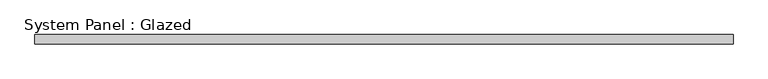
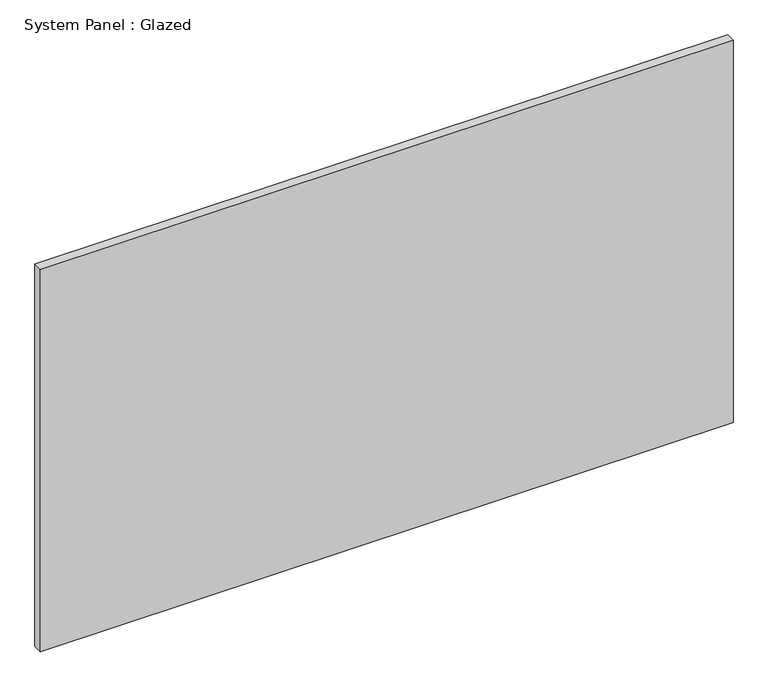
"""IFC4 building model written with IfcOpenShell, lengths in millimetres: plate geometry, System Panel : Glazed."""

from ifc_helpers import new_model, si_unit, origin, origin_with_axes, place, context, project, spatial, polyline, outline, extrude, source, transform, mapped, element, save


def system_panel_glazed_aa91312f(model_context):
    return source(origin(), model_context, "Body", "SweptSolid", [
        extrude(outline(polyline([(913.7999998, 24.5), (-913.7999998, 24.5), (-913.7999998, 49.5), (913.7999998, 49.5), (913.7999998, 24.5)])), origin_with_axes(), (0.0, 0.0, 1.0), 1066.8),
    ])


if __name__ == "__main__":
    model = new_model("IFC4")
    model_context = context("Model", 3, world=origin())
    ifc_project = project(units=[si_unit("LENGTHUNIT", "METRE", prefix="MILLI")], contexts=[model_context])
    site = spatial("IfcSite", under=ifc_project)
    building = spatial("IfcBuilding", under=site)
    placement = place(None, origin())
    system_panel_glazed_shape = system_panel_glazed_aa91312f(model_context)
    element("IfcPlate", 1, ObjectType="System Panel : Glazed", at=placement, inside=building, context=model_context, shape_type="MappedRepresentation", body=[
        mapped(system_panel_glazed_shape, transform((0.0, 0.0, 0.0), x_axis=(1.0, 0.0, 0.0), y_axis=(0.0, 1.0, 0.0), z_axis=(0.0, 0.0, 1.0))),
    ])
    save(model, "model.ifc")

# Revit data of these elements
# Type "System Panel : Glazed"
#   Keynote = "H11"
#   Construction Type Id = "GSP4R"
#   Analytic Construction = "1/8 in Pilkington single glazing"
#   Visual Light Transmittance = 0.9
#   Solar Heat Gain Coefficient = 0.86
#   Heat Transfer Coefficient (U) = 6.7069 W/(m²·K)
#   Define Thermal Properties by = 1
# Element 1 (IfcPlate, "System Panel : Glazed")
#   Materials on its faces: "Glass"
# Materials
#   "Glass": class "Glass", colour RGB 0 128 192, transparency 0.9, Description = "Soda Lime Glass", Cost = 0
